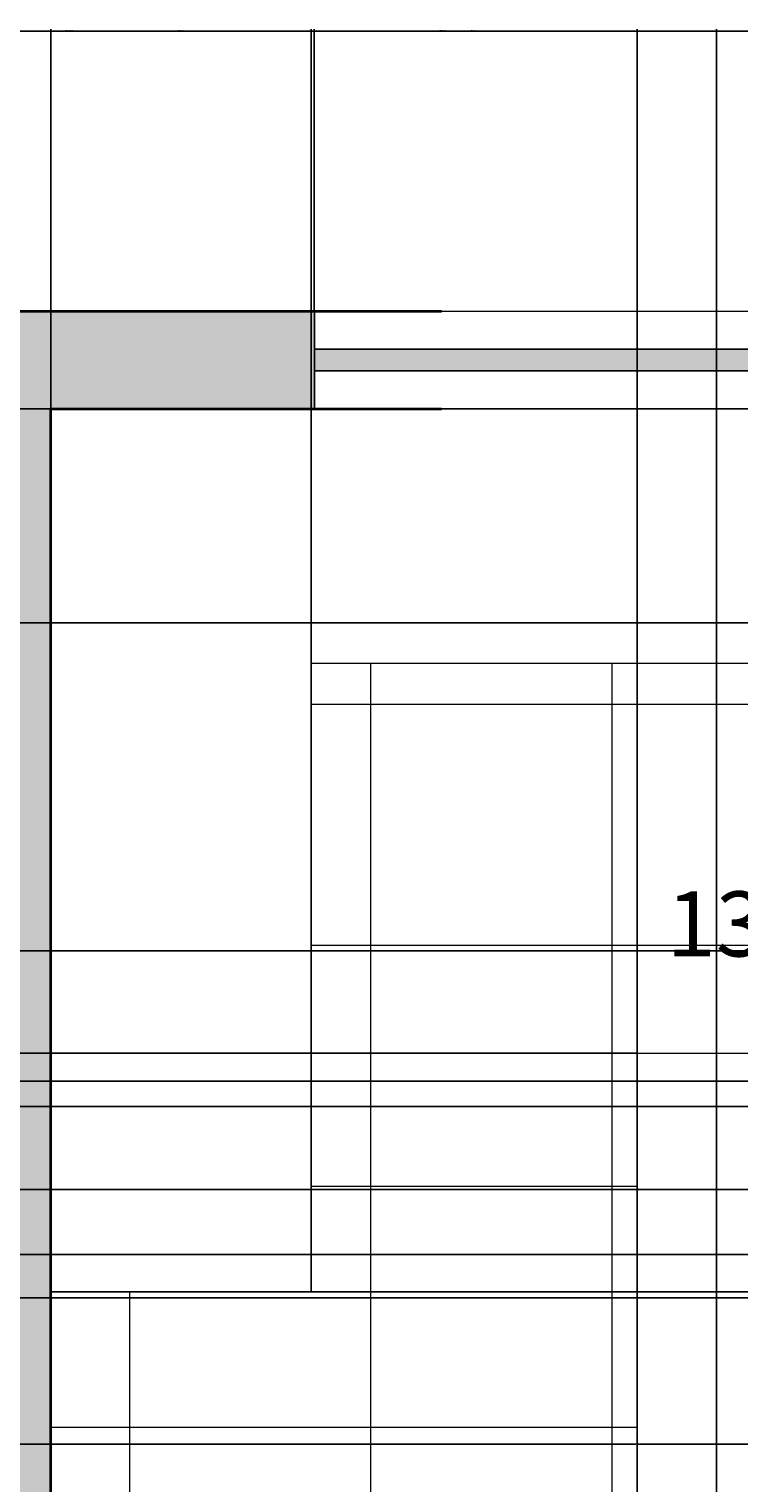
# Model space of a CAD drawing. Units: inches. Extents: x 6 to 575, y 34 to 566.
# Tile 19 of 21: x 382 to 447, y 432 to 566. Entities that reach past the tile are written whole.
import ezdxf

# ---------------------------------------------------------------- set-up
doc = ezdxf.new("R2010")
doc.units = ezdxf.units.IN
for name, color, linetype, lineweight in [('A-ANNO-DIMS', 2, 'Continuous', 18), ('A-AREA-IDEN', 6, 'Continuous', 20), ('A-FLOR-CASE', 2, 'Continuous', 18), ('A-FLOR-PATT', 252, 'Continuous', 9), ('A-GLAZ-PATT', 4, 'Continuous', 9), ('A-WALL-PATT', 251, 'Continuous', 9), ('WALLS', 7, 'Continuous', 35), ('WINDOWS', 4, 'Continuous', 20)]:
    doc.layers.add(name, color=color, linetype=linetype, lineweight=lineweight)
doc.styles.add('PDF Arial Narrow', font='txt')
doc.styles.get("Standard").update_dxf_attribs({"font": 'arial.ttf'})
doc.dimstyles.get("Standard").update_dxf_attribs({"dimtxt": 0.18, "dimasz": 0.18, "dimexe": 0.18, "dimexo": 0.0625, "dimgap": 0.09, "dimtad": 0, "dimtih": 1, "dimtoh": 1, "dimdec": 4, "dimzin": 0, "dimdsep": 46, "dimtxsty": 'Standard', "dimcen": 0.09, "dimadec": 0, "dimazin": 0, "dimtfac": 1, "dimtdec": 4, "dimtofl": 0, "dimtmove": 0, "dimatfit": 3, "dimfxl": 1, "dimtolj": 1, "dimtzin": 0, "dimarcsym": 0})

# ---------------------------------------------------------------- blocks, each defined once
blk = doc.blocks.new('WIN-48IN')
for p, q in [((0, 0), (0, 9)), ((0, 0), (0, 9)), ((0, 9), (0, 0)), ((48, 0), (48, 9)), ((0, 5.5), (48, 5.5)), ((0, 3.5), (48, 3.5))]:
    blk.add_line(p, q)
blk.add_lwpolyline([(0, 9), (48, 9), (48, 0), (0, 0)], close=True)
blk = doc.blocks.new('*D36')
at = {"layer": 'A-ANNO-DIMS', "color": 0, "lineweight": -2, "transparency": 16777216}
for p, q in [((362.66, 539.86), (362.66, 565.81)), ((362.84, 565.63), (384.83, 565.63)), ((407.76, 565.63), (385.77, 565.63)), ((407.94, 539.86), (407.94, 565.81))]:
    blk.add_line(p, q, dxfattribs=at)
at = {"layer": 'A-ANNO-DIMS', "color": 0, "transparency": 16777216}
for points in [[(362.84, 565.66), (362.84, 565.6), (362.66, 565.63)], [(407.76, 565.66), (407.76, 565.6), (407.94, 565.63)]]:
    blk.add_solid(points, dxfattribs=at)
at = {"layer": 'Defpoints', "color": 0, "transparency": 16777216}
for p in [(407.94, 565.63), (362.66, 539.8), (407.94, 539.8)]:
    blk.add_point(p, dxfattribs=at)
at = {"layer": 'A-ANNO-DIMS', "color": 0, "transparency": 16777216, "insert": (385.3, 565.63), "char_height": 0.18, "attachment_point": 5}
blk.add_mtext('\\A1;45.285', dxfattribs=at)
blk = doc.blocks.new('*D50')
at = {"layer": 'A-ANNO-DIMS', "color": 0, "lineweight": -2, "transparency": 16777216}
for p, q in [((248.7, 468.78), (574.68, 468.78)), ((574.5, 468.6), (574.5, 463.96)), ((574.5, 458.97), (574.5, 463.6)), ((248.7, 458.79), (574.68, 458.79))]:
    blk.add_line(p, q, dxfattribs=at)
at = {"layer": 'A-ANNO-DIMS', "color": 0, "transparency": 16777216}
for points in [[(574.47, 468.6), (574.53, 468.6), (574.5, 468.78)], [(574.47, 458.97), (574.53, 458.97), (574.5, 458.79)]]:
    blk.add_solid(points, dxfattribs=at)
at = {"layer": 'Defpoints', "color": 0, "transparency": 16777216}
for p in [(248.63, 468.78), (574.5, 468.78), (248.63, 458.79)]:
    blk.add_point(p, dxfattribs=at)
at = {"layer": 'A-ANNO-DIMS', "color": 0, "transparency": 16777216, "insert": (574.5, 463.78), "char_height": 0.18, "attachment_point": 5}
blk.add_mtext('\\A1;9.987', dxfattribs=at)
blk = doc.blocks.new('*D51')
at = {"layer": 'A-ANNO-DIMS', "color": 0, "lineweight": -2, "transparency": 16777216}
for p, q in [((437.69, 435.25), (437.69, 33.76)), ((485.67, 435.25), (485.67, 33.76)), ((437.87, 33.94), (461.28, 33.94)), ((485.49, 33.94), (462.08, 33.94))]:
    blk.add_line(p, q, dxfattribs=at)
at = {"layer": 'A-ANNO-DIMS', "color": 0, "transparency": 16777216}
for points in [[(437.87, 33.97), (437.87, 33.91), (437.69, 33.94)], [(485.49, 33.97), (485.49, 33.91), (485.67, 33.94)]]:
    blk.add_solid(points, dxfattribs=at)
at = {"layer": 'Defpoints', "color": 0, "transparency": 16777216}
for p in [(437.69, 435.31), (485.67, 435.31), (485.67, 33.94)]:
    blk.add_point(p, dxfattribs=at)
at = {"layer": 'A-ANNO-DIMS', "color": 0, "transparency": 16777216, "insert": (461.68, 33.94), "char_height": 0.18, "attachment_point": 5}
blk.add_mtext('\\A1;47.98', dxfattribs=at)
blk = doc.blocks.new('*D52')
at = {"layer": 'A-ANNO-DIMS', "color": 0, "lineweight": -2, "transparency": 16777216}
for p, q in [((437.62, 471.35), (6.65, 471.35)), ((6.83, 471.17), (6.83, 453.51)), ((6.83, 435.49), (6.83, 453.15)), ((437.62, 435.31), (6.65, 435.31))]:
    blk.add_line(p, q, dxfattribs=at)
at = {"layer": 'A-ANNO-DIMS', "color": 0, "transparency": 16777216}
for points in [[(6.8, 471.17), (6.86, 471.17), (6.83, 471.35)], [(6.8, 435.49), (6.86, 435.49), (6.83, 435.31)]]:
    blk.add_solid(points, dxfattribs=at)
at = {"layer": 'Defpoints', "color": 0, "transparency": 16777216}
for p in [(6.83, 471.35), (437.69, 471.35), (437.69, 435.31)]:
    blk.add_point(p, dxfattribs=at)
at = {"layer": 'A-ANNO-DIMS', "color": 0, "transparency": 16777216, "insert": (6.83, 453.33), "char_height": 0.18, "attachment_point": 5}
blk.add_mtext('\\A1;36.045', dxfattribs=at)
blk = doc.blocks.new('*D53')
at = {"layer": 'A-ANNO-DIMS', "color": 0, "lineweight": -2, "transparency": 16777216}
for p, q in [((445.02, 338), (445.02, 565.81)), ((445.2, 565.63), (464.15, 565.63)), ((483.85, 565.63), (464.9, 565.63)), ((484.03, 338), (484.03, 565.81))]:
    blk.add_line(p, q, dxfattribs=at)
at = {"layer": 'A-ANNO-DIMS', "color": 0, "transparency": 16777216}
for points in [[(445.2, 565.66), (445.2, 565.6), (445.02, 565.63)], [(483.85, 565.66), (483.85, 565.6), (484.03, 565.63)]]:
    blk.add_solid(points, dxfattribs=at)
at = {"layer": 'Defpoints', "color": 0, "transparency": 16777216}
for p in [(484.03, 565.63), (445.02, 337.94), (484.03, 337.94)]:
    blk.add_point(p, dxfattribs=at)
at = {"layer": 'A-ANNO-DIMS', "color": 0, "transparency": 16777216, "insert": (464.53, 565.63), "char_height": 0.18, "attachment_point": 5}
blk.add_mtext('\\A1;39.01', dxfattribs=at)
blk = doc.blocks.new('*D61')
at = {"layer": 'A-ANNO-DIMS', "color": 0, "lineweight": -2, "transparency": 16777216}
for p, q in [((383.66, 449.41), (383.66, 565.81)), ((383.84, 565.63), (395.26, 565.63)), ((407.47, 565.63), (396.05, 565.63)), ((407.65, 449.41), (407.65, 565.81))]:
    blk.add_line(p, q, dxfattribs=at)
at = {"layer": 'A-ANNO-DIMS', "color": 0, "transparency": 16777216}
for points in [[(383.84, 565.66), (383.84, 565.6), (383.66, 565.63)], [(407.47, 565.66), (407.47, 565.6), (407.65, 565.63)]]:
    blk.add_solid(points, dxfattribs=at)
at = {"layer": 'Defpoints', "color": 0, "transparency": 16777216}
for p in [(407.65, 565.63), (383.66, 449.35), (407.65, 449.35)]:
    blk.add_point(p, dxfattribs=at)
at = {"layer": 'A-ANNO-DIMS', "color": 0, "transparency": 16777216, "insert": (395.65, 565.63), "char_height": 0.18, "attachment_point": 5}
blk.add_mtext('\\A1;23.99', dxfattribs=at)
blk = doc.blocks.new('*D64')
at = {"layer": 'A-ANNO-DIMS', "color": 0, "lineweight": -2, "transparency": 16777216}
for p, q in [((354.721145, 452.800984), (574.675816, 452.800984)), ((574.495816, 452.620984), (574.495816, 450.980984)), ((574.495816, 448.980984), (574.495816, 450.620984)), ((354.721145, 448.800984), (574.675816, 448.800984))]:
    blk.add_line(p, q, dxfattribs=at)
at = {"layer": 'A-ANNO-DIMS', "color": 0, "transparency": 16777216}
for points in [[(574.465816, 452.620984), (574.525816, 452.620984), (574.495816, 452.800984)], [(574.465816, 448.980984), (574.525816, 448.980984), (574.495816, 448.800984)]]:
    blk.add_solid(points, dxfattribs=at)
at = {"layer": 'Defpoints', "color": 0, "transparency": 16777216}
for p in [(354.658645, 452.800984), (574.495816, 452.800984), (354.658645, 448.800984)]:
    blk.add_point(p, dxfattribs=at)
at = {"layer": 'A-ANNO-DIMS', "color": 0, "transparency": 16777216, "insert": (574.495816, 450.800984), "char_height": 0.18, "attachment_point": 5}
blk.add_mtext('\\A1;4', dxfattribs=at)
blk = doc.blocks.new('*D150')
at = {"layer": 'A-ANNO-DIMS', "color": 0, "lineweight": -2, "transparency": 16777216}
for p, q in [((407.65, 449.41), (407.65, 565.81)), ((407.83, 565.63), (422.27, 565.63)), ((437.51, 565.63), (423.06, 565.63)), ((437.69, 435.37), (437.69, 565.81))]:
    blk.add_line(p, q, dxfattribs=at)
at = {"layer": 'A-ANNO-DIMS', "color": 0, "transparency": 16777216}
for points in [[(407.83, 565.66), (407.83, 565.6), (407.65, 565.63)], [(437.51, 565.66), (437.51, 565.6), (437.69, 565.63)]]:
    blk.add_solid(points, dxfattribs=at)
at = {"layer": 'Defpoints', "color": 0, "transparency": 16777216}
for p in [(437.69, 565.63), (407.65, 449.35), (437.69, 435.31)]:
    blk.add_point(p, dxfattribs=at)
at = {"layer": 'A-ANNO-DIMS', "color": 0, "transparency": 16777216, "insert": (422.67, 565.63), "char_height": 0.18, "attachment_point": 5}
blk.add_mtext('\\A1;30.04', dxfattribs=at)
blk = doc.blocks.new('*D151')
at = {"layer": 'A-ANNO-DIMS', "color": 0, "lineweight": -2, "transparency": 16777216}
for p, q in [((437.75, 435.31), (574.68, 435.31)), ((574.5, 435.13), (574.5, 421.25)), ((574.5, 407.01), (574.5, 420.89)), ((433.77, 406.83), (574.68, 406.83))]:
    blk.add_line(p, q, dxfattribs=at)
at = {"layer": 'A-ANNO-DIMS', "color": 0, "transparency": 16777216}
for points in [[(574.47, 435.13), (574.53, 435.13), (574.5, 435.31)], [(574.47, 407.01), (574.53, 407.01), (574.5, 406.83)]]:
    blk.add_solid(points, dxfattribs=at)
at = {"layer": 'Defpoints', "color": 0, "transparency": 16777216}
for p in [(437.69, 435.31), (433.71, 406.83), (574.5, 406.83)]:
    blk.add_point(p, dxfattribs=at)
at = {"layer": 'A-ANNO-DIMS', "color": 0, "transparency": 16777216, "insert": (574.5, 421.07), "char_height": 0.18, "attachment_point": 5}
blk.add_mtext('\\A1;28.48', dxfattribs=at)
blk = doc.blocks.new('*D152')
at = {"layer": 'A-ANNO-DIMS', "color": 0, "lineweight": -2, "transparency": 16777216}
for p, q in [((383.72, 530.8), (574.68, 530.8)), ((574.5, 530.62), (574.5, 490.26)), ((574.5, 449.53), (574.5, 489.89)), ((383.72, 449.35), (574.68, 449.35))]:
    blk.add_line(p, q, dxfattribs=at)
at = {"layer": 'A-ANNO-DIMS', "color": 0, "transparency": 16777216}
for points in [[(574.47, 530.62), (574.53, 530.62), (574.5, 530.8)], [(574.47, 449.53), (574.53, 449.53), (574.5, 449.35)]]:
    blk.add_solid(points, dxfattribs=at)
at = {"layer": 'Defpoints', "color": 0, "transparency": 16777216}
for p in [(383.66, 530.8), (574.5, 530.8), (383.66, 449.35)]:
    blk.add_point(p, dxfattribs=at)
at = {"layer": 'A-ANNO-DIMS', "color": 0, "transparency": 16777216, "insert": (574.5, 490.08), "char_height": 0.18, "attachment_point": 5}
blk.add_mtext('\\A1;81.45', dxfattribs=at)
blk = doc.blocks.new('*D166')
at = {"layer": 'A-ANNO-DIMS', "color": 0, "lineweight": -2, "transparency": 16777216}
for p, q in [((383.66, 530.86), (383.66, 565.81)), ((383.84, 565.63), (419.41, 565.63)), ((455.76, 565.63), (420.19, 565.63)), ((455.94, 530.86), (455.94, 565.81))]:
    blk.add_line(p, q, dxfattribs=at)
at = {"layer": 'A-ANNO-DIMS', "color": 0, "transparency": 16777216}
for points in [[(383.84, 565.66), (383.84, 565.6), (383.66, 565.63)], [(455.76, 565.66), (455.76, 565.6), (455.94, 565.63)]]:
    blk.add_solid(points, dxfattribs=at)
at = {"layer": 'Defpoints', "color": 0, "transparency": 16777216}
for p in [(455.94, 565.63), (383.66, 530.8), (455.94, 530.8)]:
    blk.add_point(p, dxfattribs=at)
at = {"layer": 'A-ANNO-DIMS', "color": 0, "transparency": 16777216, "insert": (419.8, 565.63), "char_height": 0.18, "attachment_point": 5}
blk.add_mtext('\\A1;72.28', dxfattribs=at)
blk = doc.blocks.new('*D191')
at = {"layer": 'A-ANNO-DIMS', "color": 0, "lineweight": -2, "transparency": 16777216}
for p, q in [((374.72, 530.8), (574.68, 530.8)), ((574.5, 530.62), (574.5, 521.11)), ((574.5, 511.24), (574.5, 520.75)), ((353.8, 511.06), (574.68, 511.06))]:
    blk.add_line(p, q, dxfattribs=at)
at = {"layer": 'A-ANNO-DIMS', "color": 0, "transparency": 16777216}
for points in [[(574.47, 530.62), (574.53, 530.62), (574.5, 530.8)], [(574.47, 511.24), (574.53, 511.24), (574.5, 511.06)]]:
    blk.add_solid(points, dxfattribs=at)
at = {"layer": 'Defpoints', "color": 0, "transparency": 16777216}
for p in [(374.66, 530.8), (353.73, 511.06), (574.5, 511.06)]:
    blk.add_point(p, dxfattribs=at)
at = {"layer": 'A-ANNO-DIMS', "color": 0, "transparency": 16777216, "insert": (574.5, 520.93), "char_height": 0.18, "attachment_point": 5}
blk.add_mtext('\\A1;19.74', dxfattribs=at)
blk = doc.blocks.new('*D194')
at = {"layer": 'A-ANNO-DIMS', "color": 0, "lineweight": -2, "transparency": 16777216}
for p, q in [((374.72, 480.81), (574.68, 480.81)), ((574.5, 480.63), (574.5, 466.99)), ((574.5, 452.98), (574.5, 466.62)), ((356.78, 452.8), (574.68, 452.8))]:
    blk.add_line(p, q, dxfattribs=at)
at = {"layer": 'A-ANNO-DIMS', "color": 0, "transparency": 16777216}
for points in [[(574.47, 480.63), (574.53, 480.63), (574.5, 480.81)], [(574.47, 452.98), (574.53, 452.98), (574.5, 452.8)]]:
    blk.add_solid(points, dxfattribs=at)
at = {"layer": 'Defpoints', "color": 0, "transparency": 16777216}
for p in [(374.66, 480.81), (574.5, 480.81), (356.71, 452.8)]:
    blk.add_point(p, dxfattribs=at)
at = {"layer": 'A-ANNO-DIMS', "color": 0, "transparency": 16777216, "insert": (574.5, 466.81), "char_height": 0.18, "attachment_point": 5}
blk.add_mtext('\\A1;28.01', dxfattribs=at)
blk = doc.blocks.new('*D195')
at = {"layer": 'A-ANNO-DIMS', "color": 0, "lineweight": -2, "transparency": 16777216}
for p, q in [((364.6, 466.43), (574.68, 466.43)), ((574.5, 466.25), (574.5, 459.8)), ((574.5, 452.98), (574.5, 459.44)), ((374.72, 452.8), (574.68, 452.8))]:
    blk.add_line(p, q, dxfattribs=at)
at = {"layer": 'A-ANNO-DIMS', "color": 0, "transparency": 16777216}
for points in [[(574.47, 466.25), (574.53, 466.25), (574.5, 466.43)], [(574.47, 452.98), (574.53, 452.98), (574.5, 452.8)]]:
    blk.add_solid(points, dxfattribs=at)
at = {"layer": 'Defpoints', "color": 0, "transparency": 16777216}
for p in [(364.54, 466.43), (574.5, 466.43), (374.66, 452.8)]:
    blk.add_point(p, dxfattribs=at)
at = {"layer": 'A-ANNO-DIMS', "color": 0, "transparency": 16777216, "insert": (574.5, 459.62), "char_height": 0.18, "attachment_point": 5}
blk.add_mtext('\\A1;13.632', dxfattribs=at)
blk = doc.blocks.new('*D217')
at = {"layer": 'A-ANNO-DIMS', "color": 0, "lineweight": -2, "transparency": 16777216}
for p, q in [((408.01, 534.3), (574.68, 534.3)), ((574.5, 534.12), (574.5, 532.73)), ((574.5, 530.98), (574.5, 532.37)), ((408.01, 530.8), (574.68, 530.8))]:
    blk.add_line(p, q, dxfattribs=at)
at = {"layer": 'A-ANNO-DIMS', "color": 0, "transparency": 16777216}
for points in [[(574.47, 534.12), (574.53, 534.12), (574.5, 534.3)], [(574.47, 530.98), (574.53, 530.98), (574.5, 530.8)]]:
    blk.add_solid(points, dxfattribs=at)
at = {"layer": 'Defpoints', "color": 0, "transparency": 16777216}
for p in [(407.94, 534.3), (574.5, 534.3), (407.94, 530.8)]:
    blk.add_point(p, dxfattribs=at)
at = {"layer": 'A-ANNO-DIMS', "color": 0, "transparency": 16777216, "insert": (574.5, 532.55), "char_height": 0.18, "attachment_point": 5}
blk.add_mtext('\\A1;3.5', dxfattribs=at)
blk = doc.blocks.new('*D218')
at = {"layer": 'A-ANNO-DIMS', "color": 0, "lineweight": -2, "transparency": 16777216}
for p, q in [((408.01, 536.3), (574.68, 536.3)), ((574.5, 536.12), (574.5, 535.48)), ((574.5, 534.48), (574.5, 535.12)), ((408.01, 534.3), (574.68, 534.3))]:
    blk.add_line(p, q, dxfattribs=at)
at = {"layer": 'A-ANNO-DIMS', "color": 0, "transparency": 16777216}
for points in [[(574.47, 536.12), (574.53, 536.12), (574.5, 536.3)], [(574.47, 534.48), (574.53, 534.48), (574.5, 534.3)]]:
    blk.add_solid(points, dxfattribs=at)
at = {"layer": 'Defpoints', "color": 0, "transparency": 16777216}
for p in [(407.94, 536.3), (574.5, 536.3), (407.94, 534.3)]:
    blk.add_point(p, dxfattribs=at)
at = {"layer": 'A-ANNO-DIMS', "color": 0, "transparency": 16777216, "insert": (574.5, 535.3), "char_height": 0.18, "attachment_point": 5}
blk.add_mtext('\\A1;2', dxfattribs=at)

msp = doc.modelspace()

# ---------------------------------------------------------------- hatches: boundary and pattern name
at = {"layer": 'A-FLOR-PATT'}
h = msp.add_hatch(dxfattribs=at)
h.set_pattern_fill('NET', color=256, scale=7)
h.set_pattern_definition([(0, (-98.035, 170.147), (0, 22.225), []), (90, (-98.035, 170.147), (-22.225, 1e-15), [])])
h.paths.add_polyline_path([(539.6586, 366.801), (539.6586, 378.801), (433.708, 378.801), (383.6586, 378.801), (383.6586, 278.801), (383.6586, 224.801), (383.6586, 212.801), (407.6586, 212.801), (515.6586, 212.801), (539.6586, 212.801), (539.6586, 270.801)])
h.paths.add_polyline_path([(434.8003, 333.3365), (436.6727, 333.3365), (436.6727, 331.9322), (445.0208, 331.9322), (445.0208, 337.9397), (456.1776, 337.9397), (456.1776, 346.2878), (454.7733, 346.2878), (454.7733, 348.1603), (474.2782, 348.1603), (474.2782, 346.2878), (472.8738, 346.2878), (472.8738, 337.9397), (484.0307, 337.9397), (484.0307, 331.9322), (492.3788, 331.9322), (492.3788, 333.3365), (494.2512, 333.3365), (494.2512, 313.8316), (492.3788, 313.8316), (492.3788, 315.158), (484.0307, 315.158), (484.0307, 307.278), (492.3788, 307.278), (492.3788, 308.6823), (494.2512, 308.6823), (494.2512, 289.1774), (492.3788, 289.1774), (492.3788, 290.5818), (484.0307, 290.5818), (484.0307, 282.7018), (492.3788, 282.7018), (492.3788, 284.1062), (494.2512, 284.1062), (494.2512, 264.6013), (492.3788, 264.6013), (492.3788, 266.0056), (484.0307, 266.0056), (484.0307, 259.9201), (472.8738, 259.9201), (472.8738, 251.572), (474.2782, 251.572), (474.2782, 249.6995), (454.7733, 249.6995), (454.7733, 251.572), (456.1776, 251.572), (456.1776, 259.9201), (445.0208, 259.9201), (445.0208, 266.0056), (436.6727, 266.0056), (436.6727, 264.6013), (434.8003, 264.6013), (434.8003, 284.1062), (436.6727, 284.1062), (436.6727, 282.7018), (445.0208, 282.7018), (445.0208, 290.5818), (436.6727, 290.5818), (436.6727, 289.1774), (434.8003, 289.1774), (434.8003, 308.6823), (436.6727, 308.6823), (436.6727, 307.278), (445.0208, 307.278), (445.0208, 315.158), (436.6727, 315.158), (436.6727, 313.8316), (434.8003, 313.8316)], flags=16)
h.paths.add_polyline_path([(532.9619, 436.5144), (533.9192, 437.0672), (533.9307, 437.0472, -0.12106636), (546.2274, 440.0689), (539.6586, 440.801), (539.6586, 450.6781), (515.7066, 450.6781), (515.7066, 507.3203), (407.6494, 507.3203), (407.6494, 449.3517), (383.6586, 449.3517), (383.6586, 382.801), (433.708, 382.801), (433.708, 406.831), (539.6586, 406.831), (539.6586, 412.801), (545.7108, 412.801), (545.7108, 414.4327)])
h.paths.add_polyline_path([(437.687, 435.3082), (437.687, 471.3533), (485.6691, 471.3533), (485.6691, 435.3082)], flags=16)
at = {"layer": 'A-GLAZ-PATT'}
h = msp.add_hatch(color=256, dxfattribs=at)
h.dxf.hatch_style = 1
h.paths.add_polyline_path([(36.1586, 224.801), (38.1586, 224.801), (38.1586, 272.801), (36.1586, 272.801)])
h.paths.add_polyline_path([(167.6586, 207.301), (167.6586, 209.301), (71.6586, 209.301), (71.6586, 207.301)])
h.paths.add_polyline_path([(264.6586, 219.301), (264.6586, 221.301), (246.6586, 221.301), (246.6586, 219.301)])
h.paths.add_polyline_path([(316.6586, 221.301), (316.6586, 219.301), (334.6586, 219.301), (334.6586, 221.301)])
h.paths.add_polyline_path([(515.6586, 207.301), (515.6586, 209.301), (407.6586, 209.301), (407.6586, 207.301)])
h.paths.add_polyline_path([(543.1586, 270.801), (545.1586, 270.801), (545.1586, 366.801), (543.1586, 366.801)])
h.paths.add_polyline_path([(407.9436, 536.301), (407.9436, 534.301), (455.9436, 534.301), (455.9436, 536.301)])
h.paths.add_polyline_path([(272.6586, 536.301), (272.6586, 534.301), (320.6586, 534.301), (320.6586, 536.301)])
at = {"layer": 'A-WALL-PATT'}
h = msp.add_hatch(color=256, dxfattribs=at)
h.dxf.hatch_style = 1
h.paths.add_polyline_path([(160.6586, 539.801), (32.6586, 539.801), (32.6586, 272.801), (41.6586, 272.801), (41.6586, 286.0643), (41.6586, 358.0764), (41.6586, 379.0637), (41.6586, 407.7709), (41.6194, 407.7709), (41.6194, 431.801), (82.8918, 431.801), (82.8918, 440.801), (65.6494, 440.801), (65.6494, 440.7732), (41.6194, 440.7732), (41.6194, 515.5941), (41.6586, 530.801), (117.6586, 530.801), (117.6586, 474.801), (120.6068, 474.801), (121.6586, 474.801), (121.6586, 530.801), (137.4275, 530.801), (137.4275, 530.8356), (141.2505, 530.8356), (160.6586, 530.801)])
h.paths.add_polyline_path([(71.6586, 212.801), (41.6586, 212.801), (41.6586, 224.801), (32.6586, 224.801), (32.6586, 203.801), (71.6586, 203.801)])
h.paths.add_polyline_path([(206.6586, 215.801), (246.6586, 215.801), (246.6586, 224.801), (206.6586, 224.801), (206.6586, 230.801), (201.8157, 230.801), (197.6586, 230.801), (197.6586, 212.801), (167.6586, 212.801), (167.6586, 203.801), (206.6586, 203.801)])
h.paths.add_polyline_path([(383.6586, 224.801), (334.6586, 224.801), (334.6586, 215.801), (374.6586, 215.801), (374.6586, 203.801), (384.0753, 203.801), (407.6586, 203.801), (407.6586, 212.801), (383.6586, 212.801)])
h.paths.add_polyline_path([(548.6586, 270.801), (539.6586, 270.801), (539.6586, 212.801), (515.6586, 212.801), (515.6586, 203.801), (548.6586, 203.801)])
h.paths.add_polyline_path([(548.6586, 412.801), (545.7108, 412.801), (539.6586, 412.801), (539.6586, 382.801), (433.708, 382.801), (433.708, 378.801), (539.6586, 378.801), (539.6586, 366.801), (548.6586, 366.801)])
h.paths.add_polyline_path([(548.6586, 539.801), (455.9436, 539.801), (455.9436, 530.801), (539.6586, 530.801), (539.6586, 440.801), (548.6586, 440.801)])
h.paths.add_polyline_path([(407.9436, 539.801), (362.6586, 539.801), (362.6586, 530.801), (374.6586, 530.801), (374.6586, 452.801), (354.6586, 452.801), (354.6586, 448.801), (374.6586, 448.801), (374.6586, 278.801), (383.6586, 278.801), (383.6586, 530.801), (407.9436, 530.801)])
h.paths.add_polyline_path([(338.6586, 539.801), (320.6586, 539.801), (320.6586, 530.801), (322.6586, 530.801), (322.6586, 448.801), (326.6586, 448.801), (326.6586, 530.801), (338.6586, 530.801)])
h.paths.add_polyline_path([(272.6586, 539.801), (184.6586, 539.801), (184.6586, 530.801), (197.6586, 530.801), (197.6586, 440.801), (176.6714, 440.801), (121.6586, 440.801), (121.6586, 446.801), (117.6586, 446.801), (117.6586, 440.801), (111.6586, 440.801), (111.6586, 431.801), (197.6586, 431.801), (197.6586, 407.7709), (197.6586, 276.801), (206.6586, 276.801), (206.6586, 530.801), (272.6586, 530.801)])

# ---------------------------------------------------------------- linework, layer by layer
at = {"layer": 'A-FLOR-CASE'}
msp.add_lwpolyline([(383.6586, 449.3517), (407.6494, 449.3517), (407.6494, 507.3203), (515.7066, 507.3203), (515.7066, 450.6781), (539.6586, 450.6781)], dxfattribs=at)
msp.add_lwpolyline([(437.687, 471.3533), (485.6691, 471.3533), (485.6691, 435.3082), (437.687, 435.3082)], close=True, dxfattribs=at)
at = {"layer": 'WALLS'}
for p, q in [((362.6586, 539.801), (419.6586, 539.801)), ((383.6586, 530.801), (419.6586, 530.801)), ((383.6586, 530.801), (419.6586, 530.801)), ((383.6586, 278.801), (383.6586, 530.801))]:
    msp.add_line(p, q, dxfattribs=at)

# ---------------------------------------------------------------- block references
at = {"layer": 'WINDOWS'}
msp.add_blockref('WIN-48IN', (407.9439, 530.801), dxfattribs=at)

# ---------------------------------------------------------------- texts
at = {"layer": 'A-AREA-IDEN', "insert": (440.4003, 482.5041), "char_height": 6.000503, "attachment_point": 4, "style": 'PDF Arial Narrow'}
msp.add_mtext('13\'-0" X 12\'-4"', dxfattribs=at)

# ---------------------------------------------------------------- dimensions: what is measured, and where the dimension line sits
at = {"layer": 'A-ANNO-DIMS'}
for base, p1, p2, override, picture, middle in [((407.9436, 565.631), (362.6586, 539.801), (407.9436, 539.801), {"dimdec": 3, "dimlfac": 1, "dimrnd": 0, "dimzin": 0, "dimdsep": 46, "dimlunit": 2}, '*D36', (385.3011, 565.631)), ((407.6494, 565.631), (383.6586, 449.3517), (407.6494, 449.3517), {"dimdec": 2, "dimlfac": 1, "dimrnd": 0, "dimzin": 0, "dimdsep": 46, "dimlunit": 2}, '*D61', (395.654, 565.631)), ((455.94359, 565.63098), (383.65864, 530.80098), (455.94359, 530.80098), {"dimdec": 2, "dimlfac": 1, "dimrnd": 0, "dimzin": 0, "dimdsep": 46, "dimlunit": 2}, '*D166', (419.80112, 565.63098)), ((437.687, 565.631), (407.6494, 449.3517), (437.687, 435.3082), {"dimdec": 2, "dimlfac": 1, "dimrnd": 0, "dimzin": 0, "dimdsep": 46, "dimlunit": 2}, '*D150', (422.6682, 565.631)), ((484.0307, 565.631), (445.0208, 337.9397), (484.0307, 337.9397), {"dimdec": 2, "dimlfac": 1, "dimrnd": 0, "dimzin": 0, "dimdsep": 46, "dimlunit": 2}, '*D53', (464.5257, 565.631)), ((485.6691, 33.9447), (437.687, 435.3082), (485.6691, 435.3082), {"dimdec": 2, "dimlfac": 1, "dimrnd": 0, "dimzin": 0, "dimdsep": 46, "dimlunit": 2}, '*D51', (461.678, 33.9447))]:
    dim = msp.add_linear_dim(base=base, p1=p1, p2=p2, dimstyle='Standard', override=override, dxfattribs=at)
    dim.commit()
    dim.dimension.update_dxf_attribs({"geometry": picture, "text_midpoint": middle})
for base, p1, p2, override, picture, middle in [((574.4958, 536.301), (407.9436, 534.301), (407.9436, 536.301), {"dimdec": 0, "dimlfac": 1, "dimrnd": 0, "dimzin": 0, "dimdsep": 46, "dimlunit": 2}, '*D218', (574.4958, 535.301)), ((574.4958, 534.301), (407.9436, 530.801), (407.9436, 534.301), {"dimdec": 1, "dimlfac": 1, "dimrnd": 0, "dimzin": 0, "dimdsep": 46, "dimlunit": 2}, '*D217', (574.4958, 532.551)), ((574.4958, 511.0628), (374.6586, 530.801), (353.7344, 511.0628), {"dimdec": 2, "dimlfac": 1, "dimrnd": 0, "dimzin": 0, "dimdsep": 46, "dimlunit": 2}, '*D191', (574.4958, 520.9319)), ((574.4958, 530.801), (383.6586, 449.3517), (383.6586, 530.801), {"dimdec": 2, "dimlfac": 1, "dimrnd": 0, "dimzin": 0, "dimdsep": 46, "dimlunit": 2}, '*D152', (574.4958, 490.0764)), ((574.4958, 480.81), (356.7141, 452.801), (374.6586, 480.81), {"dimdec": 2, "dimlfac": 1, "dimrnd": 0, "dimzin": 0, "dimdsep": 46, "dimlunit": 2}, '*D194', (574.4958, 466.8055)), ((6.8286, 471.3533), (437.687, 435.3082), (437.687, 471.3533), {"dimdec": 3, "dimlfac": 1, "dimrnd": 0, "dimzin": 0, "dimdsep": 46, "dimlunit": 2}, '*D52', (6.8286, 453.3307)), ((574.49582, 468.77538), (248.6332, 458.78887), (248.6332, 468.77538), {"dimdec": 3, "dimlfac": 1, "dimrnd": 0, "dimzin": 0, "dimdsep": 46, "dimlunit": 2}, '*D50', (574.49582, 463.78213)), ((574.4958, 466.433), (374.6586, 452.801), (364.5396, 466.433), {"dimdec": 3, "dimlfac": 1, "dimrnd": 0, "dimzin": 0, "dimdsep": 46, "dimlunit": 2}, '*D195', (574.4958, 459.617)), ((574.4958, 452.801), (354.6586, 448.801), (354.6586, 452.801), {"dimdec": 0, "dimlfac": 1, "dimrnd": 0, "dimzin": 0, "dimdsep": 46, "dimlunit": 2}, '*D64', (574.4958, 450.801)), ((574.4958, 406.831), (437.687, 435.3082), (433.708, 406.831), {"dimdec": 2, "dimlfac": 1, "dimrnd": 0, "dimzin": 0, "dimdsep": 46, "dimlunit": 2}, '*D151', (574.4958, 421.0696))]:
    dim = msp.add_linear_dim(base=base, p1=p1, p2=p2, angle=90, dimstyle='Standard', override=override, dxfattribs=at)
    dim.commit()
    dim.dimension.update_dxf_attribs({"geometry": picture, "text_midpoint": middle})

doc.saveas('drawing.dxf')
